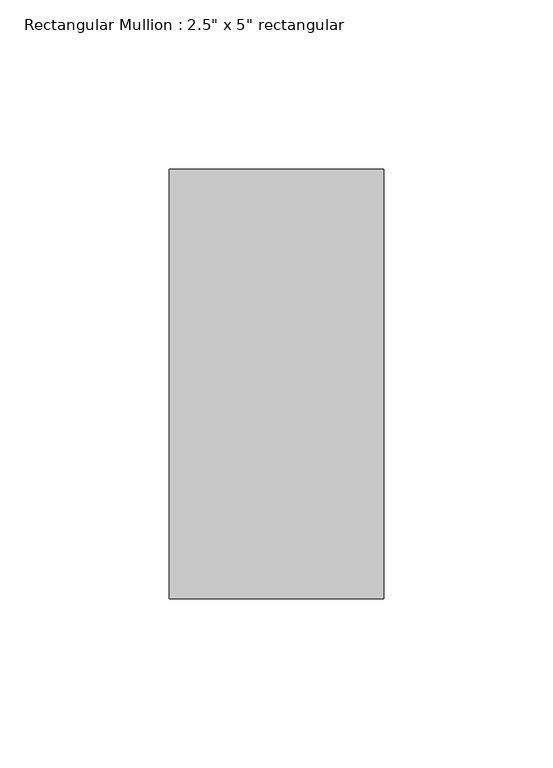
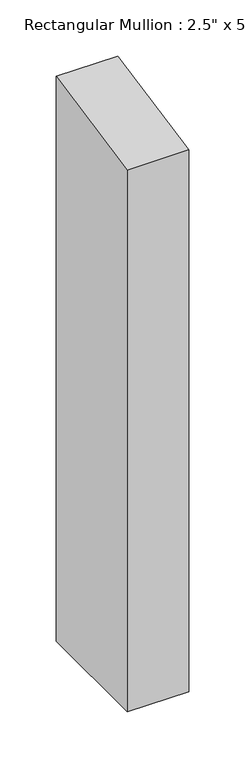
"""IFC4 building model written with IfcOpenShell, lengths in millimetres: member geometry."""

from ifc_helpers import new_model, si_unit, frame, origin, place, context, project, spatial, polyline, outline, extrude, source, transform, mapped, element, save


def member_ad26f02d(model_context):
    return source(origin(), model_context, "Body", "SweptSolid", [
        extrude(outline(polyline([(-63.5, -12.6309353), (63.5, 12.6309353), (63.5, -602.9273751), (-63.5, -602.9273751), (-63.5, -12.6309353)])), frame((-63.5, 0.0, 0.0), z_axis=(1.0, 0.0, 0.0), x_axis=(0.0, 1.0, 0.0)), (0.0, 0.0, 1.0), 63.5),
    ])


if __name__ == "__main__":
    model = new_model("IFC4")
    model_context = context("Model", 3, world=origin())
    ifc_project = project(units=[si_unit("LENGTHUNIT", "METRE", prefix="MILLI")], contexts=[model_context])
    site = spatial("IfcSite", under=ifc_project)
    building = spatial("IfcBuilding", under=site)
    placement = place(None, origin())
    member_shape = member_ad26f02d(model_context)
    element("IfcMember", 1, ObjectType="Rectangular Mullion : 2.5\" x 5\" rectangular", at=placement, inside=building, context=model_context, shape_type="MappedRepresentation", body=[
        mapped(member_shape, transform((0.0, 0.0, 0.0), x_axis=(1.0, 0.0, 0.0), y_axis=(0.0, 1.0, 0.0), z_axis=(0.0, 0.0, 1.0))),
    ])
    save(model, "model.ifc")

# Revit data of these elements
# Type "Rectangular Mullion : 2.5\" x 5\" rectangular"
#   built-in parameter 1007304 = 0.416667 (stored number, unit not read)
#   built-in parameter 1007301 = 0.104167 (stored number, unit not read)
#   built-in parameter 1007300 = 0.104167 (stored number, unit not read)
# Element 1 (IfcMember, "Rectangular Mullion : 2.5\" x 5\" rectangular")
#   Materials on its faces: "Iron, Ductile"
# Materials
#   "Iron, Ductile": class "Metal", colour RGB 0 0 0, transparency 0, Description = "Ductile cast iron", Cost = 0
